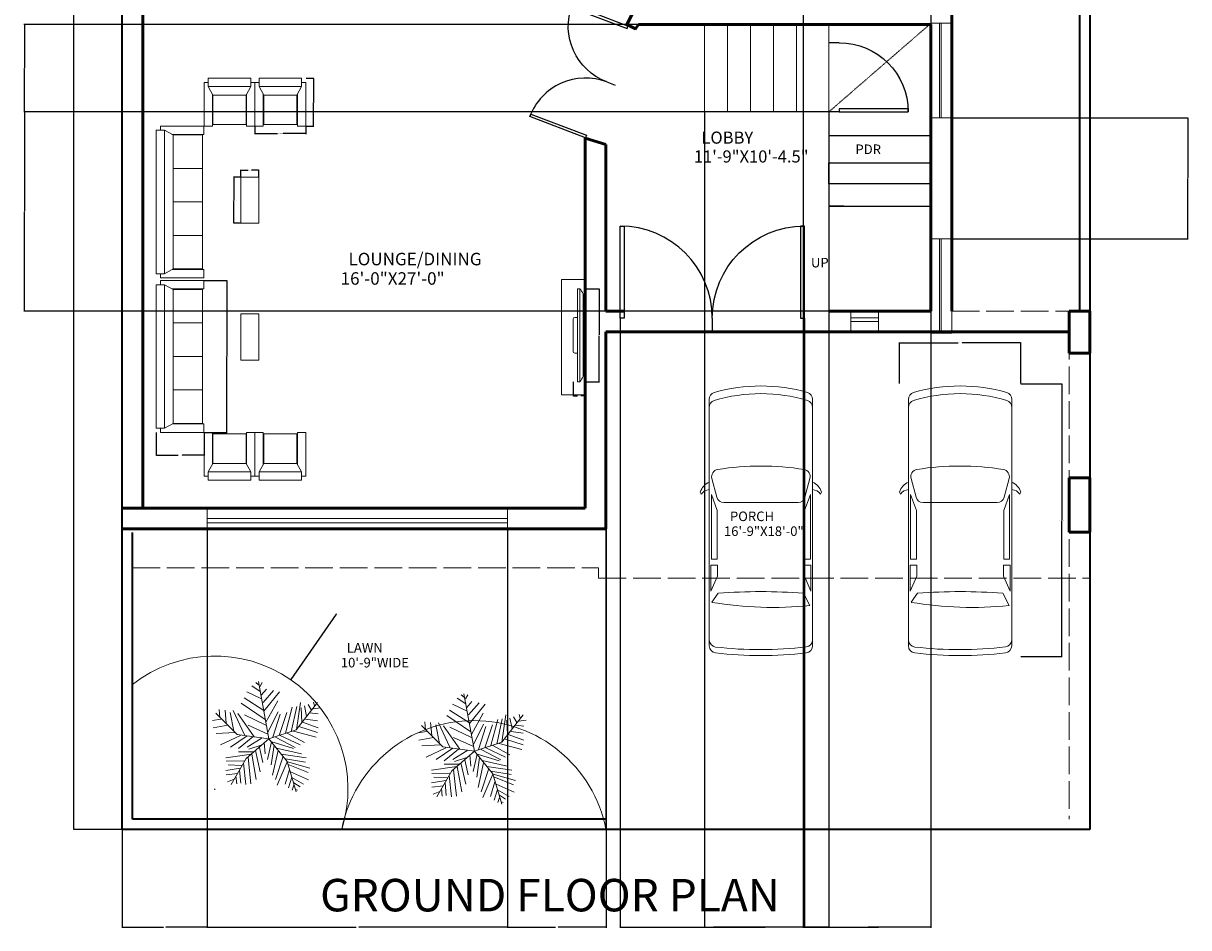
# Model space of a CAD drawing. Units: inches. Extents: x -44 to 461, y -6 to 860.
# Tile 1 of 7: x -44 to 461, y -6 to 387. Entities that reach past the tile are written whole.
import ezdxf

# ---------------------------------------------------------------- set-up
doc = ezdxf.new("R2010")
doc.units = ezdxf.units.IN
doc.header["$MEASUREMENT"] = 0
doc.linetypes.add('ACAD_ISO02W100', pattern=[15, 12, -3])
doc.linetypes.add('HIDDEN', pattern=[0.375, 0.25, -0.125])
for name, color, linetype, lineweight in [('A-ANNO-DIMS', 2, 'Continuous', 18), ('A-ANNO-TEXT', 7, 'Continuous', 18), ('A-AREA-IDEN', 7, 'Continuous', 18), ('A-COLS', 8, 'Continuous', 50), ('A-DOOR', 4, 'Continuous', 25), ('A-EQPM', 8, 'Continuous', 18), ('A-FLOR-OVHD', 8, 'ACAD_ISO02W100', 18), ('A-FLOR-STRS', 7, 'Continuous', 25), ('A-FLOR-STRS-OVHD', 7, 'HIDDEN', 18), ('C-PRKG-VEHI', 9, 'Continuous', 13), ('C-PROP', 7, 'Continuous', 35), ('furniture', 30, 'Continuous', 18), ('L-PLNT', 94, 'Continuous', 13), ('L-SITE-EDGE', 94, 'Continuous', 18), ('PLUMBING FIXTURES', 8, 'Continuous', 18), ('walls', 8, 'Continuous', 50), ('windows', 171, 'Continuous', 18)]:
    doc.layers.add(name, color=color, linetype=linetype, lineweight=lineweight)
doc.styles.get("Standard").update_dxf_attribs({"font": 'arial.ttf'})
doc.dimstyles.get("Standard").update_dxf_attribs({"dimtxt": 0.18, "dimasz": 0.18, "dimexe": 0.18, "dimexo": 0.0625, "dimgap": 0.09, "dimtad": 0, "dimtih": 1, "dimtoh": 1, "dimdec": 4, "dimzin": 0, "dimdsep": 46, "dimtxsty": 'Standard', "dimcen": 0.09, "dimadec": 0, "dimazin": 0, "dimtfac": 1, "dimtdec": 4, "dimtofl": 0, "dimtmove": 0, "dimatfit": 3, "dimfxl": 1, "dimtolj": 1, "dimtzin": 0, "dimarcsym": 0})

# ---------------------------------------------------------------- blocks, each defined once
blk = doc.blocks.new('PLASMA-LARGE')
at = {"layer": 'furniture'}
for p, q in [((-7.26, 0), (7.26, 0)), ((-21, -2.5), (21, -2.5)), ((-21, -2.5), (-21, -3.5)), ((-21, -3.5), (21, -3.5)), ((-18.61, -1), (18.61, -1)), ((-8, -1), (-8, -0.74)), ((-8, -3.5), (-8, -4.76)), ((8, -1), (8, -0.74)), ((8, -3.5), (8, -4.76)), ((21, -2.5), (21, -3.5)), ((-7.26, -5.5), (7.26, -5.5))]:
    blk.add_line(p, q, dxfattribs=at)
for centre, radius, start, end in [((-7.26, -0.74), 0.744, 90, 180), ((7.26, -0.74), 0.744, 0, 90), ((-13.97, -11.05), 11.07, 114.7602, 129.4175), ((-7.26, -4.76), 0.744, 180, 270), ((7.26, -4.76), 0.744, 270, 0), ((13.97, -11.05), 11.07, 50.5825, 65.2398)]:
    blk.add_arc(centre, radius, start, end, dxfattribs=at)
blk = doc.blocks.new('*U12')
for p, q in [((0, 0), (0, -6)), ((40, 0), (40, -6))]:
    blk.add_line(p, q)
blk.add_lwpolyline([(0, 0), (0, 40), (1.75, 40), (1.75, 0)], close=True)
blk.add_arc((0, 0), 40, 0, 90)
blk = doc.blocks.new('FABRIC SOFA 4S')
at = {"layer": 'furniture'}
for p, q in [((0, -51), (0, 51)), ((6, 51), (0, 51)), ((3, 54), (34, 54)), ((3, 51), (3, 54)), ((6, -51), (6, 51)), ((12, 47.63), (6, 51)), ((34, 48), (34, 54)), ((11.14, 48), (34, 48)), ((33, 23.81), (12, 23.81)), ((33, 0), (12, 0)), ((33, -23.81), (12, -23.81)), ((6, -51), (12, -47.63)), ((11.54, -48), (34, -48)), ((34, -48), (34, -54)), ((6, -51), (0, -51)), ((3, -54), (3, -51)), ((3, -54), (34, -54))]:
    blk.add_line(p, q, dxfattribs=at)
blk.add_lwpolyline([(12, -47.63), (12, 47.63), (33, 47.63), (33, -47.63)], close=True, dxfattribs=at)
blk = doc.blocks.new('FABRIC SOFA 1S')
at = {"layer": 'furniture'}
for p, q in [((3, 18.12), (34, 18.12)), ((3, 15.12), (3, 18.12)), ((34, 12.12), (34, 18.12)), ((0, -15.12), (0, 15.12)), ((6, 15.12), (0, 15.12)), ((6, -15.12), (6, 15.12)), ((12, 11.75), (6, 15.12)), ((11.33, 12.12), (34, 12.12)), ((6, -15.12), (0, -15.12)), ((3, -18.12), (3, -15.12)), ((6, -15.12), (12, -11.75)), ((11.33, -12.12), (34, -12.12)), ((34, -12.12), (34, -18.12)), ((3, -18.12), (34, -18.12))]:
    blk.add_line(p, q, dxfattribs=at)
blk.add_lwpolyline([(12, -11.75), (12, 11.75), (33, 11.75), (33, -11.75)], close=True, dxfattribs=at)
blk = doc.blocks.new('CAR')
at = {"layer": 'PLUMBING FIXTURES', "ltscale": 3}
for p, q in [((220804.47, -93720.06), (220804.47, -93547.3)), ((220876.86, -93720.06), (220876.86, -93547.35)), ((220870.5, -93584.17), (220875, -93575.44)), ((220810.83, -93584.17), (220806.31, -93577.76)), ((220810.23, -93596.08), (220805.58, -93585.68)), ((220805.58, -93585.68), (220805.58, -93603.85)), ((220871.11, -93596.08), (220875.75, -93585.68)), ((220875.75, -93585.68), (220875.75, -93603.85)), ((220810.23, -93603.85), (220810.23, -93596.08)), ((220871.11, -93603.85), (220871.11, -93596.08)), ((220805.58, -93603.85), (220810.23, -93603.85)), ((220805.99, -93608.09), (220810.13, -93608.09)), ((220805.99, -93653.29), (220805.99, -93608.09)), ((220810.13, -93608.09), (220810.13, -93642.08)), ((220875.75, -93603.85), (220871.11, -93603.85)), ((220875.35, -93608.09), (220871.21, -93608.09)), ((220871.21, -93608.09), (220871.21, -93642.08)), ((220875.35, -93653.29), (220875.35, -93608.09)), ((220810.13, -93642.08), (220805.99, -93653.29)), ((220814.66, -93647.63), (220866.67, -93647.63)), ((220871.21, -93642.08), (220875.35, -93653.29)), ((220798.82, -93653.49), (220798.11, -93655.1)), ((220806.3, -93664.61), (220809.78, -93651.39)), ((220875.03, -93664.61), (220871.56, -93651.39)), ((220882.52, -93653.49), (220883.22, -93655.1))]:
    blk.add_line(p, q, dxfattribs=at)
for centre, radius, start, end in [((220809.52, -93547.3), 5.05, 97.35661, 179.99999), ((220840.49, -93811.75), 271.3, 83.23106, 96.6925), ((220871.81, -93547.35), 5.05, 359.99999, 82.55935), ((220809.52, -93551.44), 5.05, 97.35661, 179.99999), ((220840.49, -93815.88), 271.3, 83.23106, 96.6925), ((220871.81, -93551.49), 5.05, 359.99999, 82.55935), ((220849.45, -93836.99), 262.8, 84.42019, 99.44802), ((220840.67, -93184.08), 401.19, 265.73533, 274.26465), ((220814.66, -93652.68), 5.05, 89.99999, 165.25643), ((220866.67, -93652.68), 5.05, 14.74356, 89.99999), ((220809.44, -93651.03), 12.03, 199.79435, 245.64582), ((220804.88, -93649.65), 7.17, 212.34744, 266.77131), ((220876.46, -93649.65), 7.17, 273.22867, 327.65255), ((220871.9, -93651.03), 12.03, 294.35417, 340.20564), ((220811.18, -93665.89), 5.05, 165.25643, 260.06484), ((220870.15, -93665.89), 5.05, 279.93514, 14.74356), ((220840.67, -93484.81), 188.52, 260.73418, 279.2658), ((220809.52, -93714.44), 5.05, 179.99999, 251.46365), ((220871.81, -93714.44), 5.05, 288.53634, 359.99999), ((220809.52, -93720.06), 5.05, 179.99999, 252.55068), ((220840.67, -93611.64), 112.45, 253.06746, 286.93252), ((220871.81, -93720.06), 5.05, 287.4493, 359.99999), ((220840.67, -93610.47), 118.98, 254.06731, 285.93267)]:
    blk.add_arc(centre, radius, start, end, dxfattribs=at)
blk = doc.blocks.new('*U17')
for p, q in [((-7.288, 39.707), (-21.778, 46.673)), ((-8.737, 47.138), (-17.069, 52.711)), ((-10.186, 53.64), (-13.084, 55.962)), ((0, 0), (-10.5, 57)), ((-9.099, 51.782), (-6.563, 55.962)), ((-7.65, 43.423), (-2.578, 49.46)), ((-5.839, 35.992), (4.667, 48.067)), ((-5.114, 27.632), (10.463, 46.673)), ((-3.665, 19.273), (-27.574, 35.527)), ((-5.114, 28.097), (-24.676, 40.636)), ((-2.941, 16.486), (8.652, 37.85)), ((27, 9), (48, 36)), ((27.127, 9.056), (31.112, 35.992)), ((44.153, 36.456), (45.239, 32.741)), ((-31.5, 4.5), (-52.5, 25.5)), ((-48.585, 21.131), (-49.309, 29.026)), ((-43.513, 28.561), (-42.427, 15.558)), ((-38.442, 26.239), (-34.819, 7.663)), ((-35.544, 28.097), (-24.314, 3.947)), ((-14.533, 2.09), (-30.834, 25.31)), ((-24.314, 23.917), (-2.941, 13.7)), ((-1.129, 6.734), (9.014, 26.704)), ((3.942, 1.625), (11.187, 24.381)), ((10.101, 3.483), (17.708, 26.239)), ((16.259, 5.805), (23.142, 31.348)), ((22.055, 7.198), (27.489, 32.277)), ((31.836, 30.883), (32.561, 16.486)), ((35.096, 32.741), (37.27, 22.524)), ((38.719, 34.134), (41.979, 28.561)), ((40.53, 25.775), (48.862, 24.846)), ((43.791, 29.954), (51.036, 30.883)), ((-47.498, 19.737), (-55.83, 18.344)), ((-40.615, 13.7), (-55.105, 10.913)), ((-20.691, 13.7), (-1.129, 4.876)), ((29.662, 12.307), (48.137, 6.269)), ((33.285, 16.486), (48.862, 10.913)), ((36.183, 19.737), (48.137, 17.88)), ((-33.37, 6.269), (-52.207, 5.34)), ((-28.299, 3.483), (-47.86, -5.805)), ((-21.416, 3.018), (-38.079, -8.128)), ((0, 0), (-31.5, 4.5)), ((-15.982, 2.09), (-30.11, -9.521)), ((0, 0), (-22.5, -19.5)), ((-6.563, 1.161), (-21.416, -8.128)), ((0, 0), (27, 9)), ((0, 0), (18, -22.5)), ((6.478, 1.625), (26.04, -8.592)), ((11.187, 3.483), (30.749, -5.805)), ((18.07, 5.805), (35.096, -3.483)), ((24.229, 7.663), (46.688, 1.625)), ((-6.563, -5.805), (-19.967, -9.985)), ((-13.446, -11.378), (-8.737, -32.741)), ((-9.461, -8.592), (-6.201, -23.453)), ((-4.752, -3.483), (-3.665, -14.629)), ((2.493, -3.019), (-1.491, -20.202)), ((1.769, -2.555), (24.229, -9.521)), ((5.029, -6.27), (2.131, -25.775)), ((9.014, -11.378), (3.58, -35.992)), ((7.565, -9.056), (32.198, -14.629)), ((-17.431, -15.094), (-42.789, -18.809)), ((-24.314, -21.596), (-42.427, -22.06)), ((-22.5, -19.5), (-37.5, -45)), ((-15.257, -12.772), (-30.11, -12.772)), ((-20.691, -18.345), (-17.793, -44.352)), ((-17.069, -15.094), (-12.721, -40.172)), ((14.085, -16.951), (6.478, -40.172)), ((18.07, -22.524), (8.289, -45.745)), ((12.274, -15.094), (36.907, -18.809)), ((16.259, -19.738), (36.183, -22.989)), ((18, -22.5), (27, -52.5)), ((18.433, -22.524), (40.53, -29.026)), ((-28.299, -29.026), (-42.789, -31.348)), ((-30.834, -34.135), (-42.427, -35.528)), ((-26.849, -26.24), (-40.253, -25.775)), ((-29.023, -30.884), (-27.936, -43.887)), ((-25.038, -23.918), (-22.865, -45.281)), ((20.244, -30.419), (15.897, -44.816)), ((19.157, -25.311), (38.719, -33.206)), ((21.331, -32.741), (39.081, -40.636)), ((-34.457, -39.708), (-40.978, -42.494)), ((-32.646, -36.921), (-31.921, -44.352)), ((22.78, -37.85), (19.519, -48.532)), ((22.78, -38.314), (34.372, -44.816)), ((24.591, -45.745), (23.142, -50.854)), ((24.591, -43.423), (30.749, -47.603)), ((26.764, -49.925), (28.213, -50.854))]:
    blk.add_line(p, q)
blk = doc.blocks.new('*D19')
at = {"layer": 'A-ANNO-DIMS', "color": 0, "lineweight": -2, "transparency": 16777216}
for p, q in [((-1.62, 817.05), (-22.6, 817.05)), ((-22.42, 816.87), (-22.42, 427.23)), ((-22.42, 37.23), (-22.42, 426.87)), ((-1.62, 37.05), (-22.6, 37.05))]:
    blk.add_line(p, q, dxfattribs=at)
at = {"layer": 'A-ANNO-DIMS', "color": 0, "transparency": 16777216}
for points in [[(-22.45, 816.87), (-22.39, 816.87), (-22.42, 817.05)], [(-22.45, 37.23), (-22.39, 37.23), (-22.42, 37.05)]]:
    blk.add_solid(points, dxfattribs=at)
at = {"layer": 'Defpoints', "color": 0, "transparency": 16777216}
for p in [(-22.42, 817.05), (-1.55, 817.05), (-1.55, 37.05)]:
    blk.add_point(p, dxfattribs=at)
at = {"layer": 'A-ANNO-DIMS', "color": 0, "transparency": 16777216, "insert": (-22.42, 427.05), "char_height": 0.18, "attachment_point": 5}
blk.add_mtext('\\A1;780.0000', dxfattribs=at)
blk = doc.blocks.new('WIN-41IN-FRAME')
for p, q in [((0, 40.98), (9, 40.98)), ((0, 40.98), (0, 0)), ((3.73, 40.98), (3.73, 0)), ((4.5, 0), (4.5, 40.98)), ((9, 40.98), (9, 0)), ((9, 0), (0, 0))]:
    blk.add_line(p, q)
blk = doc.blocks.new('TABLE-SOFA-ACCENT')
for p, q in [((0, 19.98), (7.85, 19.98)), ((0, 0), (0, 19.98)), ((7.85, 19.98), (7.85, 0)), ((7.85, 0), (0, 0))]:
    blk.add_line(p, q)
blk = doc.blocks.new('*D30')
at = {"layer": 'A-ANNO-DIMS', "color": 0, "lineweight": -2, "transparency": 16777216}
for p, q in [((56.08, 342.38), (56.08, 338.95)), ((56.26, 339.13), (65.88, 339.13)), ((78.03, 339.13), (68.42, 339.13)), ((78.21, 342.38), (78.21, 338.95))]:
    blk.add_line(p, q, dxfattribs=at)
at = {"layer": 'A-ANNO-DIMS', "color": 0, "transparency": 16777216}
for points in [[(56.26, 339.16), (56.26, 339.1), (56.08, 339.13)], [(78.03, 339.16), (78.03, 339.1), (78.21, 339.13)]]:
    blk.add_solid(points, dxfattribs=at)
at = {"layer": 'Defpoints', "color": 0, "transparency": 16777216}
for p in [(56.08, 342.44), (56.08, 339.13), (78.21, 342.44)]:
    blk.add_point(p, dxfattribs=at)
at = {"layer": 'A-ANNO-DIMS', "color": 0, "transparency": 16777216, "insert": (67.15, 339.13), "char_height": 0.18, "attachment_point": 5}
blk.add_mtext('\\A1;CHAIR 22.1282 TYP.', dxfattribs=at)
blk = doc.blocks.new('*D31')
at = {"layer": 'A-ANNO-DIMS', "color": 0, "lineweight": -2, "transparency": 16777216}
for p, q in [((78.28, 363.2), (81.71, 363.2)), ((81.53, 363.02), (81.53, 353)), ((81.53, 342.62), (81.53, 352.64)), ((78.28, 342.44), (81.71, 342.44))]:
    blk.add_line(p, q, dxfattribs=at)
at = {"layer": 'A-ANNO-DIMS', "color": 0, "transparency": 16777216}
for points in [[(81.5, 363.02), (81.56, 363.02), (81.53, 363.2)], [(81.5, 342.62), (81.56, 342.62), (81.53, 342.44)]]:
    blk.add_solid(points, dxfattribs=at)
at = {"layer": 'Defpoints', "color": 0, "transparency": 16777216}
for p in [(78.21, 363.2), (78.21, 342.44), (81.53, 342.44)]:
    blk.add_point(p, dxfattribs=at)
at = {"layer": 'A-ANNO-DIMS', "color": 0, "transparency": 16777216, "insert": (81.53, 352.82), "char_height": 0.18, "attachment_point": 5}
blk.add_mtext('\\A1;20.7547 TYP.', dxfattribs=at)
blk = doc.blocks.new('*D32')
at = {"layer": 'A-ANNO-DIMS', "color": 0, "lineweight": -2, "transparency": 16777216}
for p, q in [((34.07, 275.38), (44.08, 275.38)), ((43.9, 275.2), (43.9, 242.6)), ((43.9, 209.63), (43.9, 242.23)), ((34.07, 209.45), (44.08, 209.45))]:
    blk.add_line(p, q, dxfattribs=at)
at = {"layer": 'A-ANNO-DIMS', "color": 0, "transparency": 16777216}
for points in [[(43.87, 275.2), (43.93, 275.2), (43.9, 275.38)], [(43.87, 209.63), (43.93, 209.63), (43.9, 209.45)]]:
    blk.add_solid(points, dxfattribs=at)
at = {"layer": 'Defpoints', "color": 0, "transparency": 16777216}
for p in [(34.01, 275.38), (43.9, 275.38), (34.01, 209.45)]:
    blk.add_point(p, dxfattribs=at)
at = {"layer": 'A-ANNO-DIMS', "color": 0, "transparency": 16777216, "insert": (43.9, 242.42), "char_height": 0.18, "attachment_point": 5}
blk.add_mtext('\\A1;SOFA 65.9267 TYP.', dxfattribs=at)
blk = doc.blocks.new('*D33')
at = {"layer": 'A-ANNO-DIMS', "color": 0, "lineweight": -2, "transparency": 16777216}
for p, q in [((13.25, 209.39), (13.25, 199.38)), ((34.01, 209.39), (34.01, 199.38)), ((13.43, 199.56), (22.79, 199.56)), ((33.83, 199.56), (24.48, 199.56))]:
    blk.add_line(p, q, dxfattribs=at)
at = {"layer": 'A-ANNO-DIMS', "color": 0, "transparency": 16777216}
for points in [[(13.43, 199.59), (13.43, 199.53), (13.25, 199.56)], [(33.83, 199.59), (33.83, 199.53), (34.01, 199.56)]]:
    blk.add_solid(points, dxfattribs=at)
at = {"layer": 'Defpoints', "color": 0, "transparency": 16777216}
for p in [(13.25, 209.45), (34.01, 209.45), (34.01, 199.56)]:
    blk.add_point(p, dxfattribs=at)
at = {"layer": 'A-ANNO-DIMS', "color": 0, "transparency": 16777216, "insert": (23.63, 199.56), "char_height": 0.18, "attachment_point": 5}
blk.add_mtext('\\A1;20.7547 TYP.', dxfattribs=at)
blk = doc.blocks.new('*D34')
at = {"layer": 'A-ANNO-DIMS', "color": 0, "lineweight": -2, "transparency": 16777216}
for p, q in [((49.92, 320.26), (46.81, 320.26)), ((46.99, 320.08), (46.99, 310.45)), ((46.99, 300.46), (46.99, 310.09)), ((49.92, 300.28), (46.81, 300.28))]:
    blk.add_line(p, q, dxfattribs=at)
at = {"layer": 'A-ANNO-DIMS', "color": 0, "transparency": 16777216}
for points in [[(46.96, 320.08), (47.02, 320.08), (46.99, 320.26)], [(46.96, 300.46), (47.02, 300.46), (46.99, 300.28)]]:
    blk.add_solid(points, dxfattribs=at)
at = {"layer": 'Defpoints', "color": 0, "transparency": 16777216}
for p in [(46.99, 320.26), (49.98, 320.26), (49.98, 300.28)]:
    blk.add_point(p, dxfattribs=at)
at = {"layer": 'A-ANNO-DIMS', "color": 0, "transparency": 16777216, "insert": (46.99, 310.27), "char_height": 0.18, "attachment_point": 5}
blk.add_mtext('\\A1;END TABLE 19.9801 TYP.', dxfattribs=at)
blk = doc.blocks.new('*D35')
at = {"layer": 'A-ANNO-DIMS', "color": 0, "lineweight": -2, "transparency": 16777216}
for p, q in [((49.98, 320.32), (49.98, 323.43)), ((50.16, 323.25), (53.14, 323.25)), ((57.65, 323.25), (54.68, 323.25)), ((57.83, 320.32), (57.83, 323.43))]:
    blk.add_line(p, q, dxfattribs=at)
at = {"layer": 'A-ANNO-DIMS', "color": 0, "transparency": 16777216}
for points in [[(50.16, 323.28), (50.16, 323.22), (49.98, 323.25)], [(57.65, 323.28), (57.65, 323.22), (57.83, 323.25)]]:
    blk.add_solid(points, dxfattribs=at)
at = {"layer": 'Defpoints', "color": 0, "transparency": 16777216}
for p in [(49.98, 320.26), (57.83, 323.25), (57.83, 320.26)]:
    blk.add_point(p, dxfattribs=at)
at = {"layer": 'A-ANNO-DIMS', "color": 0, "transparency": 16777216, "insert": (53.91, 323.25), "char_height": 0.18, "attachment_point": 5}
blk.add_mtext('\\A1;7.8500 TYP.', dxfattribs=at)
blk = doc.blocks.new('*D36')
at = {"layer": 'A-ANNO-DIMS', "color": 0, "lineweight": -2, "transparency": 16777216}
for p, q in [((199.5, 271.84), (205.69, 271.84)), ((205.51, 271.66), (205.51, 251.81)), ((205.51, 231.58), (205.51, 251.44)), ((199.51, 231.4), (205.69, 231.4))]:
    blk.add_line(p, q, dxfattribs=at)
at = {"layer": 'A-ANNO-DIMS', "color": 0, "transparency": 16777216}
for points in [[(205.54, 271.66), (205.48, 271.66), (205.51, 271.84)], [(205.54, 231.58), (205.48, 231.58), (205.51, 231.4)]]:
    blk.add_solid(points, dxfattribs=at)
at = {"layer": 'Defpoints', "color": 0, "transparency": 16777216}
for p in [(199.44, 271.84), (205.51, 271.84), (199.45, 231.4)]:
    blk.add_point(p, dxfattribs=at)
at = {"layer": 'A-ANNO-DIMS', "color": 0, "transparency": 16777216, "insert": (205.51, 251.62), "char_height": 0.18, "attachment_point": 5}
blk.add_mtext('\\A1;TV 40.4391 TYP.', dxfattribs=at)
blk = doc.blocks.new('*D37')
at = {"layer": 'A-ANNO-DIMS', "color": 0, "lineweight": -2, "transparency": 16777216}
for p, q in [((194.15, 231.34), (194.15, 225.16)), ((199.45, 231.34), (199.45, 225.16)), ((194.33, 225.34), (196.03, 225.34)), ((199.27, 225.34), (197.57, 225.34))]:
    blk.add_line(p, q, dxfattribs=at)
at = {"layer": 'A-ANNO-DIMS', "color": 0, "transparency": 16777216}
for points in [[(194.33, 225.37), (194.33, 225.31), (194.15, 225.34)], [(199.27, 225.37), (199.27, 225.31), (199.45, 225.34)]]:
    blk.add_solid(points, dxfattribs=at)
at = {"layer": 'Defpoints', "color": 0, "transparency": 16777216}
for p in [(194.15, 231.4), (199.45, 231.4), (199.45, 225.34)]:
    blk.add_point(p, dxfattribs=at)
at = {"layer": 'A-ANNO-DIMS', "color": 0, "transparency": 16777216, "insert": (196.8, 225.34), "char_height": 0.18, "attachment_point": 5}
blk.add_mtext('\\A1;5.2956 TYP.', dxfattribs=at)
blk = doc.blocks.new('*D40')
at = {"layer": 'A-ANNO-DIMS', "color": 0, "lineweight": -2, "transparency": 16777216}
for p, q in [((388.52, 230.56), (406.39, 230.56)), ((406.21, 230.38), (406.21, 171.57)), ((406.21, 112.39), (406.21, 171.2)), ((388.52, 112.21), (406.39, 112.21))]:
    blk.add_line(p, q, dxfattribs=at)
at = {"layer": 'A-ANNO-DIMS', "color": 0, "transparency": 16777216}
for points in [[(406.18, 230.38), (406.24, 230.38), (406.21, 230.56)], [(406.18, 112.39), (406.24, 112.39), (406.21, 112.21)]]:
    blk.add_solid(points, dxfattribs=at)
at = {"layer": 'Defpoints', "color": 0, "transparency": 16777216}
for p in [(388.45, 230.56), (388.45, 112.21), (406.21, 112.21)]:
    blk.add_point(p, dxfattribs=at)
at = {"layer": 'A-ANNO-DIMS', "color": 0, "transparency": 16777216, "insert": (406.21, 171.39), "char_height": 0.18, "attachment_point": 5}
blk.add_mtext('\\A1;CAR 118.3510 TYP.', dxfattribs=at)
blk = doc.blocks.new('*D41')
at = {"layer": 'A-ANNO-DIMS', "color": 0, "lineweight": -2, "transparency": 16777216}
for p, q in [((335.76, 230.62), (335.76, 248.49)), ((335.94, 248.31), (361.26, 248.31)), ((388.27, 248.31), (362.95, 248.31)), ((388.45, 230.62), (388.45, 248.49))]:
    blk.add_line(p, q, dxfattribs=at)
at = {"layer": 'A-ANNO-DIMS', "color": 0, "transparency": 16777216}
for points in [[(335.94, 248.34), (335.94, 248.28), (335.76, 248.31)], [(388.27, 248.34), (388.27, 248.28), (388.45, 248.31)]]:
    blk.add_solid(points, dxfattribs=at)
at = {"layer": 'Defpoints', "color": 0, "transparency": 16777216}
for p in [(388.45, 248.31), (335.76, 230.56), (388.45, 230.56)]:
    blk.add_point(p, dxfattribs=at)
at = {"layer": 'A-ANNO-DIMS', "color": 0, "transparency": 16777216, "insert": (362.11, 248.31), "char_height": 0.18, "attachment_point": 5}
blk.add_mtext('\\A1;52.6955 TYP.', dxfattribs=at)
blk = doc.blocks.new('*D50')
at = {"layer": 'A-ANNO-DIMS', "color": 0, "lineweight": -2, "transparency": 16777216}
for p, q in [((293.95, 562.12), (293.95, -5.53)), ((349.45, 562.12), (349.45, -5.53)), ((294.13, -5.35), (321.16, -5.35)), ((349.27, -5.35), (322.23, -5.35))]:
    blk.add_line(p, q, dxfattribs=at)
at = {"layer": 'A-ANNO-DIMS', "color": 0, "transparency": 16777216}
for points in [[(294.13, -5.32), (294.13, -5.38), (293.95, -5.35)], [(349.27, -5.32), (349.27, -5.38), (349.45, -5.35)]]:
    blk.add_solid(points, dxfattribs=at)
at = {"layer": 'Defpoints', "color": 0, "transparency": 16777216}
for p in [(293.95, 562.18), (349.45, 562.18), (349.45, -5.35)]:
    blk.add_point(p, dxfattribs=at)
at = {"layer": 'A-ANNO-DIMS', "color": 0, "transparency": 16777216, "insert": (321.7, -5.35), "char_height": 0.18, "attachment_point": 5}
blk.add_mtext('\\A1;55.5000', dxfattribs=at)
blk = doc.blocks.new('*D52')
at = {"layer": 'A-ANNO-DIMS', "color": 0, "lineweight": -2, "transparency": 16777216}
for p, q in [((305.12, 261.99), (305.12, -5.53)), ((349.45, 261.99), (349.45, -5.53)), ((305.3, -5.35), (326.74, -5.35)), ((349.27, -5.35), (327.82, -5.35))]:
    blk.add_line(p, q, dxfattribs=at)
at = {"layer": 'A-ANNO-DIMS', "color": 0, "transparency": 16777216}
for points in [[(305.3, -5.32), (305.3, -5.38), (305.12, -5.35)], [(349.27, -5.32), (349.27, -5.38), (349.45, -5.35)]]:
    blk.add_solid(points, dxfattribs=at)
at = {"layer": 'Defpoints', "color": 0, "transparency": 16777216}
for p in [(305.12, 262.05), (349.45, 262.05), (349.45, -5.35)]:
    blk.add_point(p, dxfattribs=at)
at = {"layer": 'A-ANNO-DIMS', "color": 0, "transparency": 16777216, "insert": (327.28, -5.35), "char_height": 0.18, "attachment_point": 5}
blk.add_mtext('\\A1;44.3304', dxfattribs=at)
blk = doc.blocks.new('*D55')
at = {"layer": 'A-ANNO-DIMS', "color": 0, "lineweight": -2, "transparency": 16777216}
for p, q in [((35.42, 167.49), (35.42, -5.53)), ((165.72, 167.49), (165.72, -5.53)), ((35.6, -5.35), (99.97, -5.35)), ((165.54, -5.35), (101.17, -5.35))]:
    blk.add_line(p, q, dxfattribs=at)
at = {"layer": 'A-ANNO-DIMS', "color": 0, "transparency": 16777216}
for points in [[(35.6, -5.32), (35.6, -5.38), (35.42, -5.35)], [(165.54, -5.32), (165.54, -5.38), (165.72, -5.35)]]:
    blk.add_solid(points, dxfattribs=at)
at = {"layer": 'Defpoints', "color": 0, "transparency": 16777216}
for p in [(35.42, 167.55), (165.72, 167.55), (165.72, -5.35)]:
    blk.add_point(p, dxfattribs=at)
at = {"layer": 'A-ANNO-DIMS', "color": 0, "transparency": 16777216, "insert": (100.57, -5.35), "char_height": 0.18, "attachment_point": 5}
blk.add_mtext('\\A1;130.2995', dxfattribs=at)
blk = doc.blocks.new('*D56')
at = {"layer": 'A-ANNO-DIMS', "color": 0, "lineweight": -2, "transparency": 16777216}
for p, q in [((-1.55, 167.49), (-1.55, -5.53)), ((35.42, 167.49), (35.42, -5.53)), ((-1.37, -5.35), (16.4, -5.35)), ((35.24, -5.35), (17.47, -5.35))]:
    blk.add_line(p, q, dxfattribs=at)
at = {"layer": 'A-ANNO-DIMS', "color": 0, "transparency": 16777216}
for points in [[(-1.37, -5.32), (-1.37, -5.38), (-1.55, -5.35)], [(35.24, -5.32), (35.24, -5.38), (35.42, -5.35)]]:
    blk.add_solid(points, dxfattribs=at)
at = {"layer": 'Defpoints', "color": 0, "transparency": 16777216}
for p in [(-1.55, 167.55), (35.42, 167.55), (35.42, -5.35)]:
    blk.add_point(p, dxfattribs=at)
at = {"layer": 'A-ANNO-DIMS', "color": 0, "transparency": 16777216, "insert": (16.93, -5.35), "char_height": 0.18, "attachment_point": 5}
blk.add_mtext('\\A1;36.9747', dxfattribs=at)
blk = doc.blocks.new('*D57')
at = {"layer": 'A-ANNO-DIMS', "color": 0, "lineweight": -2, "transparency": 16777216}
for p, q in [((165.72, 167.49), (165.72, -5.53)), ((208.45, 167.49), (208.45, -5.53)), ((165.9, -5.35), (186.55, -5.35)), ((208.27, -5.35), (187.62, -5.35))]:
    blk.add_line(p, q, dxfattribs=at)
at = {"layer": 'A-ANNO-DIMS', "color": 0, "transparency": 16777216}
for points in [[(165.9, -5.32), (165.9, -5.38), (165.72, -5.35)], [(208.27, -5.32), (208.27, -5.38), (208.45, -5.35)]]:
    blk.add_solid(points, dxfattribs=at)
at = {"layer": 'Defpoints', "color": 0, "transparency": 16777216}
for p in [(165.72, 167.55), (208.45, 167.55), (208.45, -5.35)]:
    blk.add_point(p, dxfattribs=at)
at = {"layer": 'A-ANNO-DIMS', "color": 0, "transparency": 16777216, "insert": (187.08, -5.35), "char_height": 0.18, "attachment_point": 5}
blk.add_mtext('\\A1;42.7258', dxfattribs=at)
blk = doc.blocks.new('*D58')
at = {"layer": 'A-ANNO-DIMS', "color": 0, "lineweight": -2, "transparency": 16777216}
for p, q in [((214.54, 252.99), (214.54, -5.53)), ((294.54, 252.99), (294.54, -5.53)), ((214.72, -5.35), (254.01, -5.35)), ((294.36, -5.35), (255.07, -5.35))]:
    blk.add_line(p, q, dxfattribs=at)
at = {"layer": 'A-ANNO-DIMS', "color": 0, "transparency": 16777216}
for points in [[(214.72, -5.32), (214.72, -5.38), (214.54, -5.35)], [(294.36, -5.32), (294.36, -5.38), (294.54, -5.35)]]:
    blk.add_solid(points, dxfattribs=at)
at = {"layer": 'Defpoints', "color": 0, "transparency": 16777216}
for p in [(214.54, 253.05), (294.54, 253.05), (294.54, -5.35)]:
    blk.add_point(p, dxfattribs=at)
at = {"layer": 'A-ANNO-DIMS', "color": 0, "transparency": 16777216, "insert": (254.54, -5.35), "char_height": 0.18, "attachment_point": 5}
blk.add_mtext('\\A1;80.0000', dxfattribs=at)
blk = doc.blocks.new('*D63')
at = {"layer": 'A-ANNO-DIMS', "color": 0, "lineweight": -2, "transparency": 16777216}
for p, q in [((358.51, 346.05), (461.03, 346.05)), ((460.85, 345.87), (460.85, 319.96)), ((460.85, 293.69), (460.85, 319.6)), ((358.51, 293.51), (461.03, 293.51))]:
    blk.add_line(p, q, dxfattribs=at)
at = {"layer": 'A-ANNO-DIMS', "color": 0, "transparency": 16777216}
for points in [[(460.82, 345.87), (460.88, 345.87), (460.85, 346.05)], [(460.82, 293.69), (460.88, 293.69), (460.85, 293.51)]]:
    blk.add_solid(points, dxfattribs=at)
at = {"layer": 'Defpoints', "color": 0, "transparency": 16777216}
for p in [(358.45, 346.05), (358.45, 293.51), (460.85, 293.51)]:
    blk.add_point(p, dxfattribs=at)
at = {"layer": 'A-ANNO-DIMS', "color": 0, "transparency": 16777216, "insert": (460.85, 319.78), "char_height": 0.18, "attachment_point": 5}
blk.add_mtext('\\A1;52.5403', dxfattribs=at)
blk = doc.blocks.new('*D66')
at = {"layer": 'A-ANNO-DIMS', "color": 0, "lineweight": -2, "transparency": 16777216}
for p, q in [((251.05, 386.55), (-44.13, 386.55)), ((-43.95, 386.37), (-43.95, 367.74)), ((-43.95, 348.75), (-43.95, 367.38)), ((251.05, 348.57), (-44.13, 348.57))]:
    blk.add_line(p, q, dxfattribs=at)
at = {"layer": 'A-ANNO-DIMS', "color": 0, "transparency": 16777216}
for points in [[(-43.98, 386.37), (-43.92, 386.37), (-43.95, 386.55)], [(-43.98, 348.75), (-43.92, 348.75), (-43.95, 348.57)]]:
    blk.add_solid(points, dxfattribs=at)
at = {"layer": 'Defpoints', "color": 0, "transparency": 16777216}
for p in [(-43.95, 386.55), (251.12, 386.55), (251.12, 348.57)]:
    blk.add_point(p, dxfattribs=at)
at = {"layer": 'A-ANNO-DIMS', "color": 0, "transparency": 16777216, "insert": (-43.95, 367.56), "char_height": 0.18, "attachment_point": 5}
blk.add_mtext('\\A1;37.9808', dxfattribs=at)
blk = doc.blocks.new('*D67')
at = {"layer": 'A-ANNO-DIMS', "color": 0, "lineweight": -2, "transparency": 16777216}
for p, q in [((251.12, 348.51), (251.12, -5.53)), ((305.12, 348.51), (305.12, -5.53)), ((251.3, -5.35), (277.58, -5.35)), ((304.94, -5.35), (278.65, -5.35))]:
    blk.add_line(p, q, dxfattribs=at)
at = {"layer": 'A-ANNO-DIMS', "color": 0, "transparency": 16777216}
for points in [[(251.3, -5.32), (251.3, -5.38), (251.12, -5.35)], [(304.94, -5.32), (304.94, -5.38), (305.12, -5.35)]]:
    blk.add_solid(points, dxfattribs=at)
at = {"layer": 'Defpoints', "color": 0, "transparency": 16777216}
for p in [(251.12, 348.57), (305.12, 348.57), (251.12, -5.35)]:
    blk.add_point(p, dxfattribs=at)
at = {"layer": 'A-ANNO-DIMS', "color": 0, "transparency": 16777216, "insert": (278.12, -5.35), "char_height": 0.18, "attachment_point": 5}
blk.add_mtext('\\A1;53.9983', dxfattribs=at)
blk = doc.blocks.new('*D68')
at = {"layer": 'A-ANNO-DIMS', "color": 0, "lineweight": -2, "transparency": 16777216}
for p, q in [((305.05, 348.57), (-44.13, 348.57)), ((-43.95, 348.39), (-43.95, 305.49)), ((-43.95, 262.23), (-43.95, 305.13)), ((305.05, 262.05), (-44.13, 262.05))]:
    blk.add_line(p, q, dxfattribs=at)
at = {"layer": 'A-ANNO-DIMS', "color": 0, "transparency": 16777216}
for points in [[(-43.98, 348.39), (-43.92, 348.39), (-43.95, 348.57)], [(-43.98, 262.23), (-43.92, 262.23), (-43.95, 262.05)]]:
    blk.add_solid(points, dxfattribs=at)
at = {"layer": 'Defpoints', "color": 0, "transparency": 16777216}
for p in [(-43.95, 348.57), (305.12, 348.57), (305.12, 262.05)]:
    blk.add_point(p, dxfattribs=at)
at = {"layer": 'A-ANNO-DIMS', "color": 0, "transparency": 16777216, "insert": (-43.95, 305.31), "char_height": 0.18, "attachment_point": 5}
blk.add_mtext('\\A1;86.5192', dxfattribs=at)
blk = doc.blocks.new('*D69')
at = {"layer": 'A-ANNO-DIMS', "color": 0, "lineweight": -2, "transparency": 16777216}
for p, q in [((91.38, 130.6), (71.73, 102.25)), ((91.56, 130.6), (91.38, 130.6)), ((38.61, 54.61), (38.79, 54.61)), ((38.7, 54.52), (38.7, 54.7))]:
    blk.add_line(p, q, dxfattribs=at)
at = {"layer": 'A-ANNO-DIMS', "color": 0, "transparency": 16777216}
blk.add_solid([(71.71, 102.27), (71.75, 102.23), (71.63, 102.1)], dxfattribs=at)
at = {"layer": 'Defpoints', "color": 0, "transparency": 16777216}
for p in [(71.63, 102.1), (38.7, 54.61)]:
    blk.add_point(p, dxfattribs=at)
at = {"layer": 'A-ANNO-DIMS', "color": 0, "transparency": 16777216, "insert": (92.18, 130.6), "char_height": 0.18, "attachment_point": 5}
blk.add_mtext('\\A1;R57.7876', dxfattribs=at)

msp = doc.modelspace()

# ---------------------------------------------------------------- linework, layer by layer
at = {"layer": 'A-COLS'}
for p, q in [((409.44568, 262.0501), (409.44568, 243.90884)), ((418.44568, 262.0501), (409.44568, 262.0501)), ((418.44568, 243.90884), (418.44568, 262.0501)), ((409.44568, 243.90884), (418.44568, 243.90884)), ((409.44568, 189.75487), (418.44568, 189.75487)), ((409.44568, 166.18558), (409.44568, 189.75487)), ((418.44568, 189.75487), (418.44568, 166.18558)), ((418.44568, 166.18558), (409.44568, 166.18558))]:
    msp.add_line(p, q, dxfattribs=at)
at = {"layer": 'A-FLOR-OVHD'}
for p, q in [((358.44568, 262.0501), (418.44568, 262.0501)), ((409.44568, 253.0501), (409.44568, 41.5501)), ((2.94568, 150.68147), (205.24483, 150.68147)), ((205.24483, 150.68147), (205.24483, 146.23218)), ((205.24483, 146.23218), (418.44568, 146.23218))]:
    msp.add_line(p, q, dxfattribs=at)
at = {"layer": 'A-FLOR-STRS'}
for p, q in [((305.11528, 386.5501), (251.117, 386.5501)), ((305.11528, 348.56927), (305.11528, 262.0501)), ((349.44568, 338.22315), (305.11528, 338.22315)), ((349.44568, 326.52669), (349.44568, 338.22315)), ((305.11528, 317.41553), (305.11528, 326.52669)), ((305.11528, 326.52669), (349.44568, 326.52669)), ((349.44568, 317.41553), (305.11528, 317.41553)), ((349.44568, 307.62103), (349.44568, 317.41553)), ((311.66669, 307.62103), (305.11528, 307.62103)), ((305.11528, 307.62103), (311.66669, 307.62103)), ((311.66669, 307.62103), (349.44568, 307.62103)), ((305.11528, 262.0501), (311.66669, 262.0501))]:
    msp.add_line(p, q, dxfattribs=at)
at = {"layer": 'A-FLOR-STRS-OVHD'}
for p, q in [((251.117, 386.5501), (251.117, 348.56927)), ((261.11808, 386.5501), (261.11808, 348.56927)), ((271.11917, 386.5501), (271.11917, 348.56927)), ((281.12025, 386.5501), (281.12025, 348.56927)), ((291.12133, 386.5501), (291.12133, 348.56927)), ((305.11528, 348.56927), (349.44568, 387.03569)), ((305.11528, 348.56927), (305.11528, 386.5501)), ((251.117, 348.56927), (305.11528, 348.56927))]:
    msp.add_line(p, q, dxfattribs=at)
at = {"layer": 'C-PROP'}
for p, q in [((-1.55432, 37.0501), (-1.55432, 817.0501)), ((418.44568, 817.0501), (418.44568, 37.0501)), ((413.94568, 752.5501), (413.94568, 262.0501)), ((-1.55432, 37.0501), (-1.55432, 166.0501)), ((2.94568, 41.5501), (2.94568, 166.0501)), ((208.44568, 41.5501), (2.94568, 41.5501)), ((418.44568, 37.0501), (-1.55432, 37.0501))]:
    msp.add_line(p, q, dxfattribs=at)
at = {"layer": 'furniture'}
msp.add_lwpolyline([(189.07543, 225.74762), (189.07149, 275.89535), (199.44371, 275.89616), (199.44766, 225.74844)], close=True, dxfattribs=at)
at = {"layer": 'L-SITE-EDGE'}
msp.add_line((208.44568, 167.5501), (208.44568, 37.0501), dxfattribs=at)
for centre, radius, start, end in [((38.70122, 54.6141), 57.7876, 342.3055581, 128.2242218), ((151.10032, 25.96898), 58.40618, 10.9367373, 169.0632627)]:
    msp.add_arc(centre, radius, start, end, dxfattribs=at)
at = {"layer": 'walls'}
for p, q in [((358.44568, 752.5501), (358.44568, 262.0501)), ((7.44568, 176.5501), (7.44568, 500.5501)), ((219.77987, 391.0501), (217.44568, 386.5501)), ((217.44568, 386.5501), (221.1769, 384.57847)), ((221.1769, 384.57847), (222.47722, 386.5501)), ((222.47722, 386.5501), (349.44568, 386.5501)), ((349.44568, 386.5501), (349.44568, 262.0501)), ((199.44568, 176.5501), (199.44568, 337.42533)), ((199.44568, 337.1844), (208.44568, 334.43646)), ((208.44568, 262.0501), (208.44568, 334.43646)), ((208.44568, 262.0501), (216.29023, 262.0501)), ((305.11528, 262.0501), (349.44568, 262.0501)), ((208.44568, 253.0501), (409.44568, 253.0501)), ((208.44568, 167.5501), (208.44568, 253.0501)), ((-1.55432, 176.5501), (199.44568, 176.5501)), ((-1.55432, 167.5501), (208.44568, 167.5501))]:
    msp.add_line(p, q, dxfattribs=at)
at = {"layer": 'windows'}
for p, q in [((314.74943, 262.0501), (314.74943, 253.0501)), ((326.73144, 262.0501), (314.74943, 262.0501)), ((314.74943, 262.0501), (314.74943, 257.5501)), ((326.73144, 259.2017), (314.74943, 259.2017)), ((326.73144, 253.0501), (326.73144, 262.0501)), ((326.73144, 257.5501), (326.73144, 259.2017)), ((314.74943, 257.5501), (326.73144, 257.5501)), ((314.74943, 253.0501), (326.73144, 253.0501)), ((35.42042, 176.5501), (35.42042, 167.5501)), ((165.7199, 176.5501), (35.42042, 176.5501)), ((35.42042, 176.5501), (35.42042, 172.0501)), ((35.42042, 172.0501), (165.7199, 172.0501)), ((165.7199, 167.5501), (165.7199, 176.5501)), ((165.7199, 172.0501), (165.7199, 170.14855)), ((165.7199, 170.14855), (35.42042, 170.14855)), ((35.42042, 167.5501), (165.7199, 167.5501))]:
    msp.add_line(p, q, dxfattribs=at)

# ---------------------------------------------------------------- block references
at = {"layer": 'A-DOOR'}
for p, xscale, yscale, zscale, rotation in [((217.96705, 385.78549), -0.6473174777509669, 0.6473174777509668, 0.6473174777509666, 69.19349462187056), ((309.61414, 348.56927), -0.7498099103642428, 0.7498099103642428, 0.7498099103642428, 270), ((199.5722, 337.37725), 0.6473174777509666, 0.6473174777509666, 0.6473174777509666, 69.19349462187061)]:
    msp.add_blockref('*U12', p, dxfattribs=dict(at, xscale=xscale, yscale=yscale, zscale=zscale, rotation=rotation))
msp.add_blockref('*U12', (214.54023, 259.0501), dxfattribs=at)
at = {"layer": 'A-DOOR', "xscale": -1}
msp.add_blockref('*U12', (294.54023, 259.0501), dxfattribs=at)
at = {"layer": 'A-EQPM', "xscale": -0.9628364592350681, "yscale": 0.9628364592350692, "zscale": 0.9628364592350692, "rotation": 270.0090205836726}
msp.add_blockref('PLASMA-LARGE', (199.44562, 251.62303), dxfattribs=at)
at = {"layer": 'C-PRKG-VEHI', "xscale": -0.6191396643141144, "yscale": 0.6191396643141144, "zscale": 0.6191396643141144, "rotation": 180}
for p in [(-136455.55447, -57802.00085), (-136369.11044, -57802.00085)]:
    msp.add_blockref('CAR', p, dxfattribs=at)
at = {"layer": 'furniture', "yscale": 0.6104321447770836, "zscale": 0.6104321447770836, "rotation": 90}
for p, xscale in [((45.07221, 363.1994), -0.6104321447770836), ((67.1485, 363.1994), -0.6104321447770836), ((45.07221, 188.69884), 0.6104321447770836), ((67.1485, 188.69884), 0.6104321447770836)]:
    msp.add_blockref('FABRIC SOFA 1S', p, dxfattribs=dict(at, xscale=xscale))
at = {"layer": 'furniture', "xscale": 0.6104321447770836, "yscale": 0.6104321447770836, "zscale": 0.6104321447770836}
for p in [(13.25344, 309.48137), (13.25344, 242.41687)]:
    msp.add_blockref('FABRIC SOFA 4S', p, dxfattribs=at)
at = {"layer": 'furniture'}
for p in [(49.983, 300.277), (49.983, 240.87404)]:
    msp.add_blockref('TABLE-SOFA-ACCENT', p, dxfattribs=at)
at = {"layer": 'L-PLNT', "xscale": 0.4381751191577558, "yscale": 0.4381751191577558, "zscale": 0.4381751191577558}
for p in [(62.19225, 76.40344), (151.4032, 71.05063)]:
    msp.add_blockref('*U17', p, dxfattribs=at)
at = {"layer": 'windows'}
for p in [(349.446, 346.05086), (349.446, 252.52583)]:
    msp.add_blockref('WIN-41IN-FRAME', p, dxfattribs=at)

# ---------------------------------------------------------------- texts
at = {"layer": 'A-ANNO-TEXT'}
for s, height, p in [('UP', 4.155577, (297.38399, 281.07338)), ('GROUND FLOOR PLAN', 14.1075375, (84.38457, 1.55094))]:
    msp.add_text(s, height=height, dxfattribs=at).set_placement(p)
at = {"layer": 'A-AREA-IDEN'}
for s, height, p in [('LOBBY', 5.260005, (249.8549, 334.78061)), ('PDR', 4.155577, (316.68321, 330.27366)), ('11\'-9"X10\'-4.5"', 5.2600052, (246.56383, 326.60642)), ('LOUNGE/DINING', 5.4222944, (96.6962, 281.98531)), ('16\'-0"X27\'-0"', 5.4222944, (93.30359, 273.55891)), ('PORCH', 4.155577, (262.23239, 170.95392)), ('16\'-9"X18\'-0"', 4.1555773, (259.63234, 164.49604)), ('LAWN', 4.155577, (95.98434, 113.90665)), ('10\'-9"WIDE', 4.155577, (93.38429, 107.44876))]:
    msp.add_text(s, height=height, dxfattribs=at).set_placement(p)

# ---------------------------------------------------------------- dimensions: what is measured, and where the dimension line sits
at = {"layer": 'A-ANNO-DIMS'}
for base, p1, p2, override, picture, middle in [((-22.41551, 817.0501), (-1.55432, 37.0501), (-1.55432, 817.0501), {"dimclrd": 0, "dimclre": 0, "dimclrt": 0}, '*D19', (-22.41551, 427.0501)), ((-43.95432, 386.5501), (251.117, 348.56927), (251.117, 386.5501), {"dimdec": 4, "dimlfac": 1, "dimrnd": 0, "dimzin": 0, "dimdsep": 46, "dimlunit": 2}, '*D66', (-43.95431, 367.55969)), ((-43.95432, 348.56927), (305.11528, 262.0501), (305.11528, 348.56927), {"dimdec": 4, "dimlfac": 1, "dimrnd": 0, "dimzin": 0, "dimdsep": 46, "dimlunit": 2}, '*D68', (-43.95431, 305.30969)), ((460.84569, 293.51066), (358.44569, 346.05097), (358.44569, 293.51066), {"dimdec": 4, "dimlfac": 1, "dimrnd": 0, "dimzin": 0, "dimdsep": 46, "dimlunit": 2}, '*D63', (460.84569, 319.78081))]:
    dim = msp.add_linear_dim(base=base, p1=p1, p2=p2, angle=90, dimstyle='Standard', override=override, dxfattribs=at)
    dim.commit()
    dim.dimension.update_dxf_attribs({"geometry": picture, "text_midpoint": middle})
for base, p1, p2, picture, middle in [((349.44569, -5.3499), (293.94569, 562.17916), (349.44569, 562.17916), '*D50', (321.69569, -5.3499)), ((251.117, -5.3499), (305.11528, 348.56927), (251.117, 348.56927), '*D67', (278.11614, -5.3499)), ((349.44569, -5.3499), (305.11528, 262.0501), (349.44569, 262.0501), '*D52', (327.28048, -5.3499)), ((294.54023, -5.3499), (214.54023, 253.0501), (294.54023, 253.0501), '*D58', (254.54023, -5.3499)), ((35.42042, -5.3499), (-1.55431, 167.5501), (35.42042, 167.5501), '*D56', (16.93305, -5.3499)), ((165.7199, -5.3499), (35.42042, 167.5501), (165.7199, 167.5501), '*D55', (100.57016, -5.3499)), ((208.44568, -5.3499), (165.7199, 167.5501), (208.44568, 167.5501), '*D57', (187.08279, -5.3499))]:
    dim = msp.add_linear_dim(base=base, p1=p1, p2=p2, dimstyle='Standard', override={"dimdec": 4, "dimlfac": 1, "dimrnd": 0, "dimzin": 0, "dimdsep": 46, "dimlunit": 2}, dxfattribs=at)
    dim.commit()
    dim.dimension.update_dxf_attribs({"geometry": picture, "text_midpoint": middle})
for base, p1, p2, angle, text, picture, middle in [((81.5318, 342.4447), (78.21258, 363.1994), (78.21258, 342.4447), 270, '<> TYP.', '*D31', (81.5318, 352.82205)), ((56.08441, 339.12548), (78.21258, 342.4447), (56.08441, 342.4447), 180, 'CHAIR <> TYP.', '*D30', (67.1485, 339.12548)), ((46.98591, 320.25702), (49.98293, 300.27691), (49.98293, 320.25702), 90, 'END TABLE <> TYP.', '*D34', (46.98591, 310.26696)), ((43.89713, 275.38021), (34.00813, 209.45354), (34.00813, 275.38021), 90, 'SOFA <> TYP.', '*D32', (43.89713, 242.41687)), ((205.50831, 271.84355), (199.44881, 231.40346), (199.44244, 271.84259), 90.0090206, 'TV <> TYP.', '*D36', (205.51149, 251.62398)), ((199.44976, 225.33759), (194.1532, 231.40263), (199.44881, 231.40346), 0.0090206, '<> TYP.', '*D37', (196.80196, 225.33718)), ((406.206703, 112.211044), (388.454047, 230.562087), (388.454047, 112.211044), 270, 'CAR <> TYP.', '*D40', (406.206703, 171.386565))]:
    dim = msp.add_linear_dim(base=base, p1=p1, p2=p2, angle=angle, text=text, dimstyle='Standard', override={"dimdec": 4, "dimlfac": 1, "dimrnd": 0, "dimzin": 0, "dimdsep": 46, "dimlunit": 2}, dxfattribs=at)
    dim.commit()
    dim.dimension.update_dxf_attribs({"geometry": picture, "text_midpoint": middle})
for base, p1, p2, picture, middle in [((57.83289, 323.25403), (49.98293, 320.25702), (57.83289, 320.25702), '*D35', (53.90791, 323.25403)), ((388.45405, 248.31474), (335.75855, 230.56209), (388.45405, 230.56209), '*D41', (362.1063, 248.31474)), ((34.00813, 199.56453), (13.25344, 209.45354), (34.00813, 209.45354), '*D33', (23.63078, 199.56453))]:
    dim = msp.add_linear_dim(base=base, p1=p1, p2=p2, text='<> TYP.', dimstyle='Standard', override={"dimdec": 4, "dimlfac": 1, "dimrnd": 0, "dimzin": 0, "dimdsep": 46, "dimlunit": 2}, dxfattribs=at)
    dim.commit()
    dim.dimension.update_dxf_attribs({"geometry": picture, "text_midpoint": middle})
dim = msp.add_radius_dim(center=(38.70122, 54.6141), mpoint=(71.62772, 102.1036), dimstyle='Standard', override={"dimdec": 4, "dimlfac": 1, "dimrnd": 0, "dimzin": 0, "dimdsep": 46, "dimlunit": 2}, dxfattribs=at)
dim.commit()
dim.dimension.update_dxf_attribs({"geometry": '*D69', "text_midpoint": (92.18325, 130.5973), "dimtype": 164})

doc.saveas('drawing.dxf')
